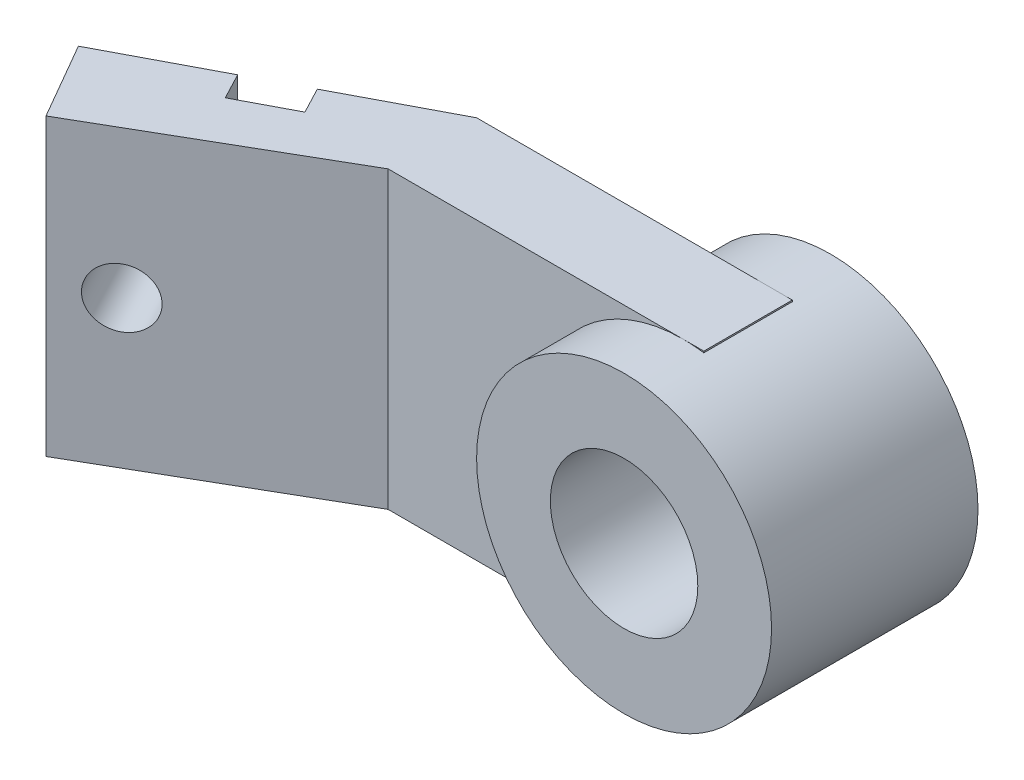
ISO-10303-21;
HEADER;
FILE_DESCRIPTION(('STEP AP214'),'2;1');
FILE_NAME('part.step','',(''),(''),'','','');
FILE_SCHEMA(('AUTOMOTIVE_DESIGN { 1 0 10303 214 1 1 1 1 }'));
ENDSEC;
DATA;
#1=APPLICATION_CONTEXT('core data for automotive mechanical design processes');
#2=APPLICATION_PROTOCOL_DEFINITION('international standard','automotive_design',2000,#1);
#3=PRODUCT_CONTEXT('',#1,'mechanical');
#4=PRODUCT('Part','Part','',(#3));
#5=PRODUCT_RELATED_PRODUCT_CATEGORY('part','',(#4));
#6=PRODUCT_DEFINITION_FORMATION('','',#4);
#7=PRODUCT_DEFINITION_CONTEXT('part definition',#1,'design');
#8=PRODUCT_DEFINITION('design','',#6,#7);
#9=PRODUCT_DEFINITION_SHAPE('','',#8);
#10=(LENGTH_UNIT() NAMED_UNIT(*) SI_UNIT(.MILLI.,.METRE.));
#11=(NAMED_UNIT(*) PLANE_ANGLE_UNIT() SI_UNIT($,.RADIAN.));
#12=(NAMED_UNIT(*) SI_UNIT($,.STERADIAN.) SOLID_ANGLE_UNIT());
#13=UNCERTAINTY_MEASURE_WITH_UNIT(LENGTH_MEASURE(1.E-05),#10,'distance_accuracy_value','');
#14=(GEOMETRIC_REPRESENTATION_CONTEXT(3) GLOBAL_UNCERTAINTY_ASSIGNED_CONTEXT((#13)) GLOBAL_UNIT_ASSIGNED_CONTEXT((#10,
#11,#12)) REPRESENTATION_CONTEXT('',''));
#15=CARTESIAN_POINT('',(0.,0.,0.));
#16=DIRECTION('',(0.,0.,1.));
#17=DIRECTION('',(1.,0.,0.));
#18=AXIS2_PLACEMENT_3D('',#15,#16,#17);
#19=CARTESIAN_POINT('',(-13.8879140481124,25.,-26.4564758559725));
#20=DIRECTION('',(-0.464788358802759,0.,-0.885421809942266));
#21=DIRECTION('',(-0.885421809942266,0.,0.464788358802759));
#22=AXIS2_PLACEMENT_3D('',#19,#20,#21);
#23=PLANE('',#22);
#24=DIRECTION('',(0.,1.,0.));
#25=VECTOR('',#24,1.);
#26=CARTESIAN_POINT('',(-67.7084361988453,-25.,1.79576717605518));
#27=LINE('',#26,#25);
#28=CARTESIAN_POINT('',(-67.7084361988453,-25.,1.79576717605518));
#29=VERTEX_POINT('',#28);
#30=CARTESIAN_POINT('',(-67.7084361988453,25.,1.79576717605518));
#31=VERTEX_POINT('',#30);
#32=EDGE_CURVE('E176',#29,#31,#27,.T.);
#33=ORIENTED_EDGE('',*,*,#32,.T.);
#34=DIRECTION('',(0.885421809942266,0.,-0.464788358802759));
#35=VECTOR('',#34,1.);
#36=CARTESIAN_POINT('',(-13.8879140481124,25.,-26.4564758559725));
#37=LINE('',#36,#35);
#38=CARTESIAN_POINT('',(-50.,25.,-7.5));
#39=VERTEX_POINT('',#38);
#40=EDGE_CURVE('E191',#31,#39,#37,.T.);
#41=ORIENTED_EDGE('',*,*,#40,.T.);
#42=DIRECTION('',(0.,-1.,0.));
#43=VECTOR('',#42,1.);
#44=CARTESIAN_POINT('',(-50.,25.,-7.5));
#45=LINE('',#44,#43);
#46=CARTESIAN_POINT('',(-50.,-25.,-7.5));
#47=VERTEX_POINT('',#46);
#48=EDGE_CURVE('E226',#39,#47,#45,.T.);
#49=ORIENTED_EDGE('',*,*,#48,.T.);
#50=DIRECTION('',(0.885421809942266,0.,-0.464788358802759));
#51=VECTOR('',#50,1.);
#52=CARTESIAN_POINT('',(-13.8879140481124,-25.,-26.4564758559725));
#53=LINE('',#52,#51);
#54=EDGE_CURVE('E214',#29,#47,#53,.T.);
#55=ORIENTED_EDGE('',*,*,#54,.F.);
#56=EDGE_LOOP('',(#33,#41,#49,#55));
#57=FACE_BOUND('',#56,.T.);
#58=ADVANCED_FACE('F43',(#57),#23,.T.);
#59=CARTESIAN_POINT('',(0.,0.,17.5));
#60=DIRECTION('',(0.,0.,1.));
#61=DIRECTION('',(1.,0.,0.));
#62=AXIS2_PLACEMENT_3D('',#59,#60,#61);
#63=PLANE('',#62);
#64=CARTESIAN_POINT('',(0.,0.,17.5));
#65=DIRECTION('',(0.,0.,1.));
#66=DIRECTION('',(1.,0.,0.));
#67=AXIS2_PLACEMENT_3D('',#64,#65,#66);
#68=CIRCLE('',#67,25.);
#69=CARTESIAN_POINT('',(25.,0.,17.5));
#70=VERTEX_POINT('',#69);
#71=EDGE_CURVE('E11',#70,#70,#68,.T.);
#72=ORIENTED_EDGE('',*,*,#71,.T.);
#73=EDGE_LOOP('',(#72));
#74=FACE_BOUND('',#73,.T.);
#75=CARTESIAN_POINT('',(0.,0.,17.5));
#76=DIRECTION('',(0.,0.,1.));
#77=DIRECTION('',(1.,0.,0.));
#78=AXIS2_PLACEMENT_3D('',#75,#76,#77);
#79=CIRCLE('',#78,12.5);
#80=CARTESIAN_POINT('',(12.5,0.,17.5));
#81=VERTEX_POINT('',#80);
#82=EDGE_CURVE('E254',#81,#81,#79,.T.);
#83=ORIENTED_EDGE('',*,*,#82,.F.);
#84=EDGE_LOOP('',(#83));
#85=FACE_BOUND('',#84,.T.);
#86=ADVANCED_FACE('F270',(#74,#85),#63,.T.);
#87=CARTESIAN_POINT('',(0.,0.,-17.5));
#88=DIRECTION('',(0.,0.,1.));
#89=DIRECTION('',(1.,0.,0.));
#90=AXIS2_PLACEMENT_3D('',#87,#88,#89);
#91=PLANE('',#90);
#92=CARTESIAN_POINT('',(0.,0.,-17.5));
#93=DIRECTION('',(0.,0.,1.));
#94=DIRECTION('',(1.,0.,0.));
#95=AXIS2_PLACEMENT_3D('',#92,#93,#94);
#96=CIRCLE('',#95,25.);
#97=CARTESIAN_POINT('',(25.,0.,-17.5));
#98=VERTEX_POINT('',#97);
#99=EDGE_CURVE('E55',#98,#98,#96,.T.);
#100=ORIENTED_EDGE('',*,*,#99,.F.);
#101=EDGE_LOOP('',(#100));
#102=FACE_BOUND('',#101,.T.);
#103=CARTESIAN_POINT('',(0.,0.,-17.5));
#104=DIRECTION('',(0.,0.,1.));
#105=DIRECTION('',(1.,0.,0.));
#106=AXIS2_PLACEMENT_3D('',#103,#104,#105);
#107=CIRCLE('',#106,12.5);
#108=CARTESIAN_POINT('',(12.5,0.,-17.5));
#109=VERTEX_POINT('',#108);
#110=EDGE_CURVE('E256',#109,#109,#107,.T.);
#111=ORIENTED_EDGE('',*,*,#110,.T.);
#112=EDGE_LOOP('',(#111));
#113=FACE_BOUND('',#112,.T.);
#114=ADVANCED_FACE('F262',(#102,#113),#91,.F.);
#115=CARTESIAN_POINT('',(0.,0.,17.5));
#116=DIRECTION('',(0.,0.,-1.));
#117=DIRECTION('',(-1.,0.,0.));
#118=AXIS2_PLACEMENT_3D('',#115,#116,#117);
#119=CYLINDRICAL_SURFACE('',#118,25.);
#120=CARTESIAN_POINT('',(0.,0.,7.49999999999999));
#121=DIRECTION('',(0.,0.,1.));
#122=DIRECTION('',(1.,0.,0.));
#123=AXIS2_PLACEMENT_3D('',#120,#121,#122);
#124=CIRCLE('',#123,25.);
#125=CARTESIAN_POINT('',(3.5205883588033,24.7508678152476,7.49999999999999));
#126=VERTEX_POINT('',#125);
#127=CARTESIAN_POINT('',(0.,25.,7.49999999999999));
#128=VERTEX_POINT('',#127);
#129=EDGE_CURVE('E255',#126,#128,#124,.T.);
#130=ORIENTED_EDGE('',*,*,#129,.T.);
#131=CARTESIAN_POINT('',(0.,-25.,7.49999999999999));
#132=VERTEX_POINT('',#131);
#133=EDGE_CURVE('E251',#128,#132,#124,.T.);
#134=ORIENTED_EDGE('',*,*,#133,.T.);
#135=CARTESIAN_POINT('',(3.5205883588033,-24.7508678152476,7.49999999999999));
#136=VERTEX_POINT('',#135);
#137=EDGE_CURVE('E248',#132,#136,#124,.T.);
#138=ORIENTED_EDGE('',*,*,#137,.T.);
#139=DIRECTION('',(0.,0.,-1.));
#140=VECTOR('',#139,1.);
#141=CARTESIAN_POINT('',(3.5205883588033,-24.7508678152476,17.5));
#142=LINE('',#141,#140);
#143=CARTESIAN_POINT('',(3.5205883588033,-24.7508678152476,-7.5));
#144=VERTEX_POINT('',#143);
#145=EDGE_CURVE('E249',#136,#144,#142,.T.);
#146=ORIENTED_EDGE('',*,*,#145,.T.);
#147=CARTESIAN_POINT('',(0.,0.,-7.5));
#148=DIRECTION('',(0.,0.,-1.));
#149=DIRECTION('',(-1.,0.,0.));
#150=AXIS2_PLACEMENT_3D('',#147,#148,#149);
#151=CIRCLE('',#150,25.);
#152=CARTESIAN_POINT('',(0.,-25.,-7.5));
#153=VERTEX_POINT('',#152);
#154=EDGE_CURVE('E245',#144,#153,#151,.T.);
#155=ORIENTED_EDGE('',*,*,#154,.T.);
#156=CARTESIAN_POINT('',(0.,25.,-7.5));
#157=VERTEX_POINT('',#156);
#158=EDGE_CURVE('E239',#153,#157,#151,.T.);
#159=ORIENTED_EDGE('',*,*,#158,.T.);
#160=CARTESIAN_POINT('',(3.5205883588033,24.7508678152476,-7.5));
#161=VERTEX_POINT('',#160);
#162=EDGE_CURVE('E241',#157,#161,#151,.T.);
#163=ORIENTED_EDGE('',*,*,#162,.T.);
#164=DIRECTION('',(0.,0.,-1.));
#165=VECTOR('',#164,1.);
#166=CARTESIAN_POINT('',(3.5205883588033,24.7508678152476,17.5));
#167=LINE('',#166,#165);
#168=EDGE_CURVE('E244',#161,#126,#167,.F.);
#169=ORIENTED_EDGE('',*,*,#168,.T.);
#170=EDGE_LOOP('',(#130,#134,#138,#146,#155,#159,#163,#169));
#171=FACE_BOUND('',#170,.T.);
#172=ORIENTED_EDGE('',*,*,#71,.F.);
#173=EDGE_LOOP('',(#172));
#174=FACE_BOUND('',#173,.T.);
#175=ORIENTED_EDGE('',*,*,#99,.T.);
#176=EDGE_LOOP('',(#175));
#177=FACE_BOUND('',#176,.T.);
#178=ADVANCED_FACE('F44',(#171,#174,#177),#119,.T.);
#179=CARTESIAN_POINT('',(0.,0.,17.5));
#180=DIRECTION('',(0.,0.,-1.));
#181=DIRECTION('',(-1.,0.,0.));
#182=AXIS2_PLACEMENT_3D('',#179,#180,#181);
#183=CYLINDRICAL_SURFACE('',#182,12.5);
#184=ORIENTED_EDGE('',*,*,#110,.F.);
#185=EDGE_LOOP('',(#184));
#186=FACE_BOUND('',#185,.T.);
#187=ORIENTED_EDGE('',*,*,#82,.T.);
#188=EDGE_LOOP('',(#187));
#189=FACE_BOUND('',#188,.T.);
#190=ADVANCED_FACE('F269',(#186,#189),#183,.F.);
#191=CARTESIAN_POINT('',(0.,25.,0.));
#192=DIRECTION('',(0.,1.,0.));
#193=DIRECTION('',(0.,0.,1.));
#194=AXIS2_PLACEMENT_3D('',#191,#192,#193);
#195=PLANE('',#194);
#196=DIRECTION('',(-0.464788358802759,0.,-0.885421809942265));
#197=VECTOR('',#196,1.);
#198=CARTESIAN_POINT('',(-65.3844944048315,25.,6.2228762257665));
#199=LINE('',#198,#197);
#200=CARTESIAN_POINT('',(-65.3844944048315,25.,6.2228762257665));
#201=VERTEX_POINT('',#200);
#202=EDGE_CURVE('E166',#201,#31,#199,.T.);
#203=ORIENTED_EDGE('',*,*,#202,.F.);
#204=DIRECTION('',(0.885421809942266,0.,-0.464788358802759));
#205=VECTOR('',#204,1.);
#206=CARTESIAN_POINT('',(-74.2387125042542,25.,10.8707598137941));
#207=LINE('',#206,#205);
#208=CARTESIAN_POINT('',(-74.2387125042542,25.,10.8707598137941));
#209=VERTEX_POINT('',#208);
#210=EDGE_CURVE('E173',#209,#201,#207,.T.);
#211=ORIENTED_EDGE('',*,*,#210,.F.);
#212=DIRECTION('',(0.464788358802759,0.,0.885421809942266));
#213=VECTOR('',#212,1.);
#214=CARTESIAN_POINT('',(-76.562654298268,25.,6.44365076408277));
#215=LINE('',#214,#213);
#216=CARTESIAN_POINT('',(-76.562654298268,25.,6.44365076408277));
#217=VERTEX_POINT('',#216);
#218=EDGE_CURVE('E149',#217,#209,#215,.T.);
#219=ORIENTED_EDGE('',*,*,#218,.F.);
#220=CARTESIAN_POINT('',(-94.2710904971133,25.,15.739417940138));
#221=VERTEX_POINT('',#220);
#222=EDGE_CURVE('E193',#221,#217,#37,.T.);
#223=ORIENTED_EDGE('',*,*,#222,.F.);
#224=DIRECTION('',(-0.500000000000002,0.,-0.866025403784438));
#225=VECTOR('',#224,1.);
#226=CARTESIAN_POINT('',(-77.5186857613048,25.,44.7554340915156));
#227=LINE('',#226,#225);
#228=CARTESIAN_POINT('',(-86.7710904971133,25.,28.7297989969045));
#229=VERTEX_POINT('',#228);
#230=EDGE_CURVE('E196',#229,#221,#227,.T.);
#231=ORIENTED_EDGE('',*,*,#230,.F.);
#232=DIRECTION('',(-0.866025403784438,0.,0.500000000000002));
#233=VECTOR('',#232,1.);
#234=CARTESIAN_POINT('',(-9.25240473580844,25.,-16.025635094611));
#235=LINE('',#234,#233);
#236=CARTESIAN_POINT('',(-50.,25.,7.5));
#237=VERTEX_POINT('',#236);
#238=EDGE_CURVE('E203',#237,#229,#235,.T.);
#239=ORIENTED_EDGE('',*,*,#238,.F.);
#240=DIRECTION('',(-1.,0.,0.));
#241=VECTOR('',#240,1.);
#242=CARTESIAN_POINT('',(0.,25.,7.49999999999999));
#243=LINE('',#242,#241);
#244=EDGE_CURVE('E189',#128,#237,#243,.T.);
#245=ORIENTED_EDGE('',*,*,#244,.F.);
#246=CARTESIAN_POINT('',(3.5205883588033,25.,7.49999999999999));
#247=VERTEX_POINT('',#246);
#248=EDGE_CURVE('E183',#247,#128,#243,.T.);
#249=ORIENTED_EDGE('',*,*,#248,.F.);
#250=DIRECTION('',(0.,0.,1.));
#251=VECTOR('',#250,1.);
#252=CARTESIAN_POINT('',(3.5205883588033,25.,0.));
#253=LINE('',#252,#251);
#254=CARTESIAN_POINT('',(3.5205883588033,25.,-7.5));
#255=VERTEX_POINT('',#254);
#256=EDGE_CURVE('E186',#255,#247,#253,.T.);
#257=ORIENTED_EDGE('',*,*,#256,.F.);
#258=DIRECTION('',(1.,0.,0.));
#259=VECTOR('',#258,1.);
#260=CARTESIAN_POINT('',(0.,25.,-7.5));
#261=LINE('',#260,#259);
#262=EDGE_CURVE('E194',#157,#255,#261,.T.);
#263=ORIENTED_EDGE('',*,*,#262,.F.);
#264=EDGE_CURVE('E70',#39,#157,#261,.T.);
#265=ORIENTED_EDGE('',*,*,#264,.F.);
#266=ORIENTED_EDGE('',*,*,#40,.F.);
#267=EDGE_LOOP('',(#203,#211,#219,#223,#231,#239,#245,#249,#257,#263,#265,#266));
#268=FACE_BOUND('',#267,.T.);
#269=ADVANCED_FACE('F272',(#268),#195,.T.);
#270=CARTESIAN_POINT('',(0.,-25.,0.));
#271=DIRECTION('',(0.,1.,0.));
#272=DIRECTION('',(0.,0.,1.));
#273=AXIS2_PLACEMENT_3D('',#270,#271,#272);
#274=PLANE('',#273);
#275=DIRECTION('',(0.885421809942266,0.,-0.464788358802759));
#276=VECTOR('',#275,1.);
#277=CARTESIAN_POINT('',(-74.2387125042542,-25.,10.8707598137941));
#278=LINE('',#277,#276);
#279=CARTESIAN_POINT('',(-74.2387125042542,-25.,10.8707598137941));
#280=VERTEX_POINT('',#279);
#281=CARTESIAN_POINT('',(-65.3844944048315,-25.,6.2228762257665));
#282=VERTEX_POINT('',#281);
#283=EDGE_CURVE('E160',#280,#282,#278,.T.);
#284=ORIENTED_EDGE('',*,*,#283,.T.);
#285=DIRECTION('',(-0.464788358802759,0.,-0.885421809942265));
#286=VECTOR('',#285,1.);
#287=CARTESIAN_POINT('',(-65.3844944048315,-25.,6.2228762257665));
#288=LINE('',#287,#286);
#289=EDGE_CURVE('E165',#282,#29,#288,.T.);
#290=ORIENTED_EDGE('',*,*,#289,.T.);
#291=ORIENTED_EDGE('',*,*,#54,.T.);
#292=DIRECTION('',(1.,0.,0.));
#293=VECTOR('',#292,1.);
#294=CARTESIAN_POINT('',(0.,-25.,-7.5));
#295=LINE('',#294,#293);
#296=EDGE_CURVE('E215',#47,#153,#295,.T.);
#297=ORIENTED_EDGE('',*,*,#296,.T.);
#298=CARTESIAN_POINT('',(3.5205883588033,-25.,-7.5));
#299=VERTEX_POINT('',#298);
#300=EDGE_CURVE('E211',#153,#299,#295,.T.);
#301=ORIENTED_EDGE('',*,*,#300,.T.);
#302=DIRECTION('',(0.,0.,1.));
#303=VECTOR('',#302,1.);
#304=CARTESIAN_POINT('',(3.5205883588033,-25.,0.));
#305=LINE('',#304,#303);
#306=CARTESIAN_POINT('',(3.5205883588033,-25.,7.49999999999999));
#307=VERTEX_POINT('',#306);
#308=EDGE_CURVE('E208',#299,#307,#305,.T.);
#309=ORIENTED_EDGE('',*,*,#308,.T.);
#310=DIRECTION('',(-1.,0.,0.));
#311=VECTOR('',#310,1.);
#312=CARTESIAN_POINT('',(0.,-25.,7.49999999999999));
#313=LINE('',#312,#311);
#314=EDGE_CURVE('E202',#307,#132,#313,.T.);
#315=ORIENTED_EDGE('',*,*,#314,.T.);
#316=CARTESIAN_POINT('',(-50.,-25.,7.5));
#317=VERTEX_POINT('',#316);
#318=EDGE_CURVE('E185',#132,#317,#313,.T.);
#319=ORIENTED_EDGE('',*,*,#318,.T.);
#320=DIRECTION('',(-0.866025403784438,0.,0.500000000000002));
#321=VECTOR('',#320,1.);
#322=CARTESIAN_POINT('',(-9.25240473580844,-25.,-16.025635094611));
#323=LINE('',#322,#321);
#324=CARTESIAN_POINT('',(-86.7710904971133,-25.,28.7297989969045));
#325=VERTEX_POINT('',#324);
#326=EDGE_CURVE('E218',#317,#325,#323,.T.);
#327=ORIENTED_EDGE('',*,*,#326,.T.);
#328=DIRECTION('',(-0.500000000000002,0.,-0.866025403784438));
#329=VECTOR('',#328,1.);
#330=CARTESIAN_POINT('',(-77.5186857613048,-25.,44.7554340915156));
#331=LINE('',#330,#329);
#332=CARTESIAN_POINT('',(-94.2710904971133,-25.,15.739417940138));
#333=VERTEX_POINT('',#332);
#334=EDGE_CURVE('E220',#325,#333,#331,.T.);
#335=ORIENTED_EDGE('',*,*,#334,.T.);
#336=CARTESIAN_POINT('',(-76.562654298268,-25.,6.44365076408277));
#337=VERTEX_POINT('',#336);
#338=EDGE_CURVE('E169',#333,#337,#53,.T.);
#339=ORIENTED_EDGE('',*,*,#338,.T.);
#340=DIRECTION('',(0.464788358802759,0.,0.885421809942266));
#341=VECTOR('',#340,1.);
#342=CARTESIAN_POINT('',(-76.562654298268,-25.,6.44365076408277));
#343=LINE('',#342,#341);
#344=EDGE_CURVE('E58',#337,#280,#343,.T.);
#345=ORIENTED_EDGE('',*,*,#344,.T.);
#346=EDGE_LOOP('',(#284,#290,#291,#297,#301,#309,#315,#319,#327,#335,#339,#345));
#347=FACE_BOUND('',#346,.T.);
#348=ADVANCED_FACE('F164',(#347),#274,.F.);
#349=CARTESIAN_POINT('',(0.,25.,7.49999999999999));
#350=DIRECTION('',(0.,0.,1.));
#351=DIRECTION('',(1.,0.,0.));
#352=AXIS2_PLACEMENT_3D('',#349,#350,#351);
#353=PLANE('',#352);
#354=ORIENTED_EDGE('',*,*,#129,.F.);
#355=DIRECTION('',(0.,-1.,0.));
#356=VECTOR('',#355,1.);
#357=CARTESIAN_POINT('',(3.5205883588033,25.,7.49999999999999));
#358=LINE('',#357,#356);
#359=EDGE_CURVE('E237',#247,#126,#358,.T.);
#360=ORIENTED_EDGE('',*,*,#359,.F.);
#361=ORIENTED_EDGE('',*,*,#248,.T.);
#362=EDGE_LOOP('',(#354,#360,#361));
#363=FACE_BOUND('',#362,.T.);
#364=ADVANCED_FACE('F294',(#363),#353,.T.);
#365=ORIENTED_EDGE('',*,*,#133,.F.);
#366=ORIENTED_EDGE('',*,*,#244,.T.);
#367=DIRECTION('',(0.,-1.,0.));
#368=VECTOR('',#367,1.);
#369=CARTESIAN_POINT('',(-50.,25.,7.5));
#370=LINE('',#369,#368);
#371=EDGE_CURVE('E204',#237,#317,#370,.T.);
#372=ORIENTED_EDGE('',*,*,#371,.T.);
#373=ORIENTED_EDGE('',*,*,#318,.F.);
#374=EDGE_LOOP('',(#365,#366,#372,#373));
#375=FACE_BOUND('',#374,.T.);
#376=ADVANCED_FACE('F293',(#375),#353,.T.);
#377=CARTESIAN_POINT('',(3.5205883588033,25.,0.));
#378=DIRECTION('',(1.,0.,0.));
#379=DIRECTION('',(0.,0.,-1.));
#380=AXIS2_PLACEMENT_3D('',#377,#378,#379);
#381=PLANE('',#380);
#382=ORIENTED_EDGE('',*,*,#145,.F.);
#383=EDGE_CURVE('E233',#136,#307,#358,.T.);
#384=ORIENTED_EDGE('',*,*,#383,.T.);
#385=ORIENTED_EDGE('',*,*,#308,.F.);
#386=DIRECTION('',(0.,-1.,0.));
#387=VECTOR('',#386,1.);
#388=CARTESIAN_POINT('',(3.5205883588033,25.,-7.5));
#389=LINE('',#388,#387);
#390=EDGE_CURVE('E232',#144,#299,#389,.T.);
#391=ORIENTED_EDGE('',*,*,#390,.F.);
#392=EDGE_LOOP('',(#382,#384,#385,#391));
#393=FACE_BOUND('',#392,.T.);
#394=ADVANCED_FACE('F298',(#393),#381,.T.);
#395=ORIENTED_EDGE('',*,*,#168,.F.);
#396=EDGE_CURVE('E234',#255,#161,#389,.T.);
#397=ORIENTED_EDGE('',*,*,#396,.F.);
#398=ORIENTED_EDGE('',*,*,#256,.T.);
#399=ORIENTED_EDGE('',*,*,#359,.T.);
#400=EDGE_LOOP('',(#395,#397,#398,#399));
#401=FACE_BOUND('',#400,.T.);
#402=ADVANCED_FACE('F299',(#401),#381,.T.);
#403=CARTESIAN_POINT('',(0.,25.,-7.5));
#404=DIRECTION('',(0.,0.,-1.));
#405=DIRECTION('',(-1.,0.,0.));
#406=AXIS2_PLACEMENT_3D('',#403,#404,#405);
#407=PLANE('',#406);
#408=ORIENTED_EDGE('',*,*,#162,.F.);
#409=ORIENTED_EDGE('',*,*,#262,.T.);
#410=ORIENTED_EDGE('',*,*,#396,.T.);
#411=EDGE_LOOP('',(#408,#409,#410));
#412=FACE_BOUND('',#411,.T.);
#413=ADVANCED_FACE('F304',(#412),#407,.T.);
#414=ORIENTED_EDGE('',*,*,#154,.F.);
#415=ORIENTED_EDGE('',*,*,#390,.T.);
#416=ORIENTED_EDGE('',*,*,#300,.F.);
#417=EDGE_LOOP('',(#414,#415,#416));
#418=FACE_BOUND('',#417,.T.);
#419=ADVANCED_FACE('F295',(#418),#407,.T.);
#420=ORIENTED_EDGE('',*,*,#137,.F.);
#421=ORIENTED_EDGE('',*,*,#314,.F.);
#422=ORIENTED_EDGE('',*,*,#383,.F.);
#423=EDGE_LOOP('',(#420,#421,#422));
#424=FACE_BOUND('',#423,.T.);
#425=ADVANCED_FACE('F290',(#424),#353,.T.);
#426=ORIENTED_EDGE('',*,*,#158,.F.);
#427=ORIENTED_EDGE('',*,*,#296,.F.);
#428=ORIENTED_EDGE('',*,*,#48,.F.);
#429=ORIENTED_EDGE('',*,*,#264,.T.);
#430=EDGE_LOOP('',(#426,#427,#428,#429));
#431=FACE_BOUND('',#430,.T.);
#432=ADVANCED_FACE('F292',(#431),#407,.T.);
#433=CARTESIAN_POINT('',(-85.4168723976907,0.,11.0915343521104));
#434=DIRECTION('',(-0.464788358802759,0.,-0.885421809942266));
#435=DIRECTION('',(-0.885421809942266,0.,0.464788358802759));
#436=AXIS2_PLACEMENT_3D('',#433,#434,#435);
#437=CIRCLE('',#436,5.);
#438=CARTESIAN_POINT('',(-89.843981447402,0.,13.4154761461242));
#439=VERTEX_POINT('',#438);
#440=EDGE_CURVE('E174',#439,#439,#437,.T.);
#441=ORIENTED_EDGE('',*,*,#440,.F.);
#442=EDGE_LOOP('',(#441));
#443=FACE_BOUND('',#442,.T.);
#444=DIRECTION('',(0.,1.,0.));
#445=VECTOR('',#444,1.);
#446=CARTESIAN_POINT('',(-76.562654298268,-25.,6.44365076408277));
#447=LINE('',#446,#445);
#448=EDGE_CURVE('E152',#337,#217,#447,.T.);
#449=ORIENTED_EDGE('',*,*,#448,.F.);
#450=ORIENTED_EDGE('',*,*,#338,.F.);
#451=DIRECTION('',(0.,-1.,0.));
#452=VECTOR('',#451,1.);
#453=CARTESIAN_POINT('',(-94.2710904971133,25.,15.739417940138));
#454=LINE('',#453,#452);
#455=EDGE_CURVE('E228',#221,#333,#454,.T.);
#456=ORIENTED_EDGE('',*,*,#455,.F.);
#457=ORIENTED_EDGE('',*,*,#222,.T.);
#458=EDGE_LOOP('',(#449,#450,#456,#457));
#459=FACE_BOUND('',#458,.T.);
#460=ADVANCED_FACE('F287',(#443,#459),#23,.T.);
#461=CARTESIAN_POINT('',(-77.5186857613048,25.,44.7554340915156));
#462=DIRECTION('',(-0.866025403784437,0.,0.500000000000002));
#463=DIRECTION('',(0.500000000000002,0.,0.866025403784437));
#464=AXIS2_PLACEMENT_3D('',#461,#462,#463);
#465=PLANE('',#464);
#466=ORIENTED_EDGE('',*,*,#334,.F.);
#467=DIRECTION('',(0.,-1.,0.));
#468=VECTOR('',#467,1.);
#469=CARTESIAN_POINT('',(-86.7710904971133,25.,28.7297989969045));
#470=LINE('',#469,#468);
#471=EDGE_CURVE('E221',#229,#325,#470,.T.);
#472=ORIENTED_EDGE('',*,*,#471,.F.);
#473=ORIENTED_EDGE('',*,*,#230,.T.);
#474=ORIENTED_EDGE('',*,*,#455,.T.);
#475=EDGE_LOOP('',(#466,#472,#473,#474));
#476=FACE_BOUND('',#475,.T.);
#477=ADVANCED_FACE('F303',(#476),#465,.T.);
#478=CARTESIAN_POINT('',(-9.25240473580844,25.,-16.025635094611));
#479=DIRECTION('',(0.500000000000002,0.,0.866025403784438));
#480=DIRECTION('',(0.866025403784438,0.,-0.500000000000002));
#481=AXIS2_PLACEMENT_3D('',#478,#479,#480);
#482=PLANE('',#481);
#483=CARTESIAN_POINT('',(-78.626369514948,0.,24.027442145377));
#484=DIRECTION('',(0.500000000000002,0.,0.866025403784438));
#485=DIRECTION('',(0.866025403784438,0.,-0.500000000000002));
#486=AXIS2_PLACEMENT_3D('',#483,#484,#485);
#487=ELLIPSE('',#486,5.00404346790341,5.);
#488=CARTESIAN_POINT('',(-74.292740750102,0.,21.5254204114253));
#489=VERTEX_POINT('',#488);
#490=EDGE_CURVE('E50',#489,#489,#487,.T.);
#491=ORIENTED_EDGE('',*,*,#490,.F.);
#492=EDGE_LOOP('',(#491));
#493=FACE_BOUND('',#492,.T.);
#494=ORIENTED_EDGE('',*,*,#326,.F.);
#495=ORIENTED_EDGE('',*,*,#371,.F.);
#496=ORIENTED_EDGE('',*,*,#238,.T.);
#497=ORIENTED_EDGE('',*,*,#471,.T.);
#498=EDGE_LOOP('',(#494,#495,#496,#497));
#499=FACE_BOUND('',#498,.T.);
#500=ADVANCED_FACE('F310',(#493,#499),#482,.T.);
#501=CARTESIAN_POINT('',(-65.3844944048315,-25.,6.2228762257665));
#502=DIRECTION('',(0.885421809942266,0.,-0.464788358802759));
#503=DIRECTION('',(-0.464788358802759,0.,-0.885421809942266));
#504=AXIS2_PLACEMENT_3D('',#501,#502,#503);
#505=PLANE('',#504);
#506=ORIENTED_EDGE('',*,*,#202,.T.);
#507=ORIENTED_EDGE('',*,*,#32,.F.);
#508=ORIENTED_EDGE('',*,*,#289,.F.);
#509=DIRECTION('',(0.,1.,0.));
#510=VECTOR('',#509,1.);
#511=CARTESIAN_POINT('',(-65.3844944048315,-25.,6.2228762257665));
#512=LINE('',#511,#510);
#513=EDGE_CURVE('E153',#282,#201,#512,.T.);
#514=ORIENTED_EDGE('',*,*,#513,.T.);
#515=EDGE_LOOP('',(#506,#507,#508,#514));
#516=FACE_BOUND('',#515,.T.);
#517=ADVANCED_FACE('F311',(#516),#505,.F.);
#518=CARTESIAN_POINT('',(-74.2387125042542,-25.,10.8707598137941));
#519=DIRECTION('',(0.464788358802759,0.,0.885421809942266));
#520=DIRECTION('',(0.885421809942266,0.,-0.464788358802759));
#521=AXIS2_PLACEMENT_3D('',#518,#519,#520);
#522=PLANE('',#521);
#523=ORIENTED_EDGE('',*,*,#210,.T.);
#524=ORIENTED_EDGE('',*,*,#513,.F.);
#525=ORIENTED_EDGE('',*,*,#283,.F.);
#526=DIRECTION('',(0.,1.,0.));
#527=VECTOR('',#526,1.);
#528=CARTESIAN_POINT('',(-74.2387125042542,-25.,10.8707598137941));
#529=LINE('',#528,#527);
#530=EDGE_CURVE('E144',#280,#209,#529,.T.);
#531=ORIENTED_EDGE('',*,*,#530,.T.);
#532=EDGE_LOOP('',(#523,#524,#525,#531));
#533=FACE_BOUND('',#532,.T.);
#534=ADVANCED_FACE('F158',(#533),#522,.F.);
#535=CARTESIAN_POINT('',(-76.562654298268,-25.,6.44365076408277));
#536=DIRECTION('',(-0.885421809942266,0.,0.464788358802759));
#537=DIRECTION('',(0.464788358802759,0.,0.885421809942266));
#538=AXIS2_PLACEMENT_3D('',#535,#536,#537);
#539=PLANE('',#538);
#540=ORIENTED_EDGE('',*,*,#218,.T.);
#541=ORIENTED_EDGE('',*,*,#530,.F.);
#542=ORIENTED_EDGE('',*,*,#344,.F.);
#543=ORIENTED_EDGE('',*,*,#448,.T.);
#544=EDGE_LOOP('',(#540,#541,#542,#543));
#545=FACE_BOUND('',#544,.T.);
#546=ADVANCED_FACE('F150',(#545),#539,.F.);
#547=CARTESIAN_POINT('',(-54.3049709727967,0.,70.3597056577198));
#548=DIRECTION('',(-0.464788358802759,0.,-0.885421809942266));
#549=DIRECTION('',(-0.885421809942266,0.,0.464788358802759));
#550=AXIS2_PLACEMENT_3D('',#547,#548,#549);
#551=CYLINDRICAL_SURFACE('',#550,5.);
#552=ORIENTED_EDGE('',*,*,#490,.T.);
#553=EDGE_LOOP('',(#552));
#554=FACE_BOUND('',#553,.T.);
#555=ORIENTED_EDGE('',*,*,#440,.T.);
#556=EDGE_LOOP('',(#555));
#557=FACE_BOUND('',#556,.T.);
#558=ADVANCED_FACE('F325',(#554,#557),#551,.F.);
#559=CLOSED_SHELL('',(#58,#86,#114,#178,#190,#269,#348,#364,#376,#394,#402,#413,#419,#425,#432,
#460,#477,#500,#517,#534,#546,#558));
#560=MANIFOLD_SOLID_BREP('B2',#559);
#561=ADVANCED_BREP_SHAPE_REPRESENTATION('',(#18,#560),#14);
#562=SHAPE_DEFINITION_REPRESENTATION(#9,#561);
ENDSEC;
END-ISO-10303-21;
